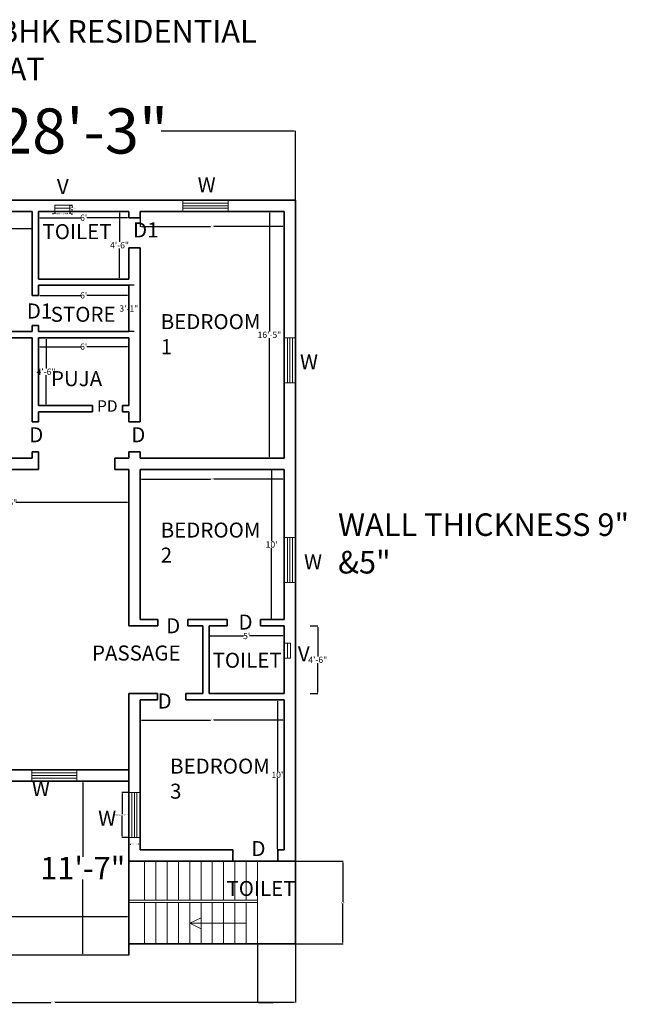
# Model space of a CAD drawing. Units: inches. Extents: x -304 to 580, y 363 to 1149.
# Tile 11 of 11: x 96 to 580, y 363 to 1149. Entities that reach past the tile are written whole.
import ezdxf

# ---------------------------------------------------------------- set-up
doc = ezdxf.new("R2010")
doc.units = ezdxf.units.IN
doc.header["$MEASUREMENT"] = 0
for name, color, linetype, lineweight in [('A-ANNO-DIMS', 2, 'Continuous', 13), ('A-ANNO-IDEN', 7, 'Continuous', 18), ('A-ANNO-SYMB', 7, 'Continuous', 18), ('A-ANNO-TEXT', 7, 'Continuous', 25), ('A-AREA-IDEN', 7, 'Continuous', 25), ('A-FLOR-OTLN', 2, 'Continuous', 25), ('A-FLOR-STRS', 40, 'Continuous', 18), ('A-GLAZ', 4, 'Continuous', 18), ('A-GLAZ-VENT', 4, 'Continuous', 18), ('A-WALL', 40, 'Continuous', 35)]:
    doc.layers.add(name, color=color, linetype=linetype, lineweight=lineweight)
doc.styles.get("Standard").update_dxf_attribs({"font": 'arial.ttf'})
doc.dimstyles.get("Standard").update_dxf_attribs({"dimtxt": 1, "dimasz": 1, "dimexe": 0.18, "dimexo": 0.0625, "dimgap": 0.09, "dimtad": 0, "dimtih": 1, "dimtoh": 1, "dimdec": 0, "dimzin": 0, "dimdsep": 46, "dimlunit": 3, "dimtxsty": 'Standard', "dimcen": 0.09, "dimadec": 0, "dimazin": 0, "dimtfac": 1, "dimtdec": 0, "dimtofl": 0, "dimtmove": 0, "dimatfit": 3, "dimfxl": 1, "dimtolj": 1, "dimtzin": 0, "dimarcsym": 0})

# ---------------------------------------------------------------- blocks, each defined once
blk = doc.blocks.new('*D2')
at = {"layer": 'A-ANNO-DIMS', "color": 0, "lineweight": -2, "transparency": 16777216}
for p, q in [((-22.57, 1005.01), (-22.57, 1060.38)), ((-21.57, 1060.2), (84.7, 1060.2)), ((315.43, 1060.2), (209.16, 1060.2)), ((316.43, 1005.01), (316.43, 1060.38))]:
    blk.add_line(p, q, dxfattribs=at)
at = {"layer": 'A-ANNO-DIMS', "color": 0, "transparency": 16777216}
for points in [[(-21.57, 1060.37), (-21.57, 1060.04), (-22.57, 1060.2)], [(315.43, 1060.37), (315.43, 1060.04), (316.43, 1060.2)]]:
    blk.add_solid(points, dxfattribs=at)
at = {"layer": 'Defpoints', "color": 0, "transparency": 16777216}
for p in [(316.43, 1060.2), (-22.57, 1004.95), (316.43, 1004.95)]:
    blk.add_point(p, dxfattribs=at)
at = {"layer": 'A-ANNO-DIMS', "color": 0, "transparency": 16777216, "insert": (146.93, 1060.2), "char_height": 1, "attachment_point": 5}
blk.add_mtext('\\A1;{\\H36x;28\'-3"}', dxfattribs=at)
blk = doc.blocks.new('*D4')
at = {"layer": 'A-ANNO-DIMS', "color": 0, "lineweight": -2, "transparency": 16777216}
for p, q in [((-13.57, 789.88), (-13.57, 763.24)), ((183.43, 789.88), (183.43, 763.24)), ((-12.57, 763.42), (76.49, 763.42)), ((182.43, 763.42), (93.37, 763.42))]:
    blk.add_line(p, q, dxfattribs=at)
at = {"layer": 'A-ANNO-DIMS', "color": 0, "transparency": 16777216}
for points in [[(-12.57, 763.59), (-12.57, 763.26), (-13.57, 763.42)], [(182.43, 763.59), (182.43, 763.26), (183.43, 763.42)]]:
    blk.add_solid(points, dxfattribs=at)
at = {"layer": 'Defpoints', "color": 0, "transparency": 16777216}
for p in [(-13.57, 789.95), (183.43, 789.95), (183.43, 763.42)]:
    blk.add_point(p, dxfattribs=at)
at = {"layer": 'A-ANNO-DIMS', "color": 0, "transparency": 16777216, "insert": (84.93, 763.42), "char_height": 1, "attachment_point": 5}
blk.add_mtext('\\A1;{\\H5x;16\'-5"}', dxfattribs=at)
blk = doc.blocks.new('*D5')
at = {"layer": 'A-ANNO-DIMS', "color": 0, "lineweight": -2, "transparency": 16777216}
for p, q in [((-13.57, 995.88), (-13.57, 981.84)), ((106.43, 995.88), (106.43, 981.84)), ((-12.57, 982.02), (42.33, 982.02)), ((105.43, 982.02), (50.53, 982.02))]:
    blk.add_line(p, q, dxfattribs=at)
at = {"layer": 'A-ANNO-DIMS', "color": 0, "transparency": 16777216}
for points in [[(-12.57, 982.19), (-12.57, 981.85), (-13.57, 982.02)], [(105.43, 982.19), (105.43, 981.85), (106.43, 982.02)]]:
    blk.add_solid(points, dxfattribs=at)
at = {"layer": 'Defpoints', "color": 0, "transparency": 16777216}
for p in [(-13.57, 995.95), (106.43, 995.95), (106.43, 982.02)]:
    blk.add_point(p, dxfattribs=at)
at = {"layer": 'A-ANNO-DIMS', "color": 0, "transparency": 16777216, "insert": (46.43, 982.02), "char_height": 1, "attachment_point": 5}
blk.add_mtext("\\A1;{\\H5x;10'}", dxfattribs=at)
blk = doc.blocks.new('*D7')
at = {"layer": 'A-ANNO-DIMS', "color": 0, "lineweight": -2, "transparency": 16777216}
for p, q in [((183.37, 995.95), (175.83, 995.95)), ((176.01, 994.95), (176.01, 971.59)), ((176.01, 942.95), (176.01, 966.3)), ((183.37, 941.95), (175.83, 941.95))]:
    blk.add_line(p, q, dxfattribs=at)
at = {"layer": 'A-ANNO-DIMS', "color": 0, "transparency": 16777216}
for points in [[(175.84, 994.95), (176.17, 994.95), (176.01, 995.95)], [(175.84, 942.95), (176.17, 942.95), (176.01, 941.95)]]:
    blk.add_solid(points, dxfattribs=at)
at = {"layer": 'Defpoints', "color": 0, "transparency": 16777216}
for p in [(183.43, 995.95), (176.01, 941.95), (183.43, 941.95)]:
    blk.add_point(p, dxfattribs=at)
at = {"layer": 'A-ANNO-DIMS', "color": 0, "transparency": 16777216, "insert": (176.01, 968.95), "char_height": 1, "attachment_point": 5}
blk.add_mtext('\\A1;{\\H5x;4\'-6"}', dxfattribs=at)
blk = doc.blocks.new('*D8')
at = {"layer": 'A-ANNO-DIMS', "color": 0, "lineweight": -2, "transparency": 16777216}
for p, q in [((111.43, 995.88), (111.43, 990.77)), ((112.43, 990.95), (145.03, 990.95)), ((182.43, 990.95), (149.83, 990.95)), ((183.43, 995.88), (183.43, 990.77))]:
    blk.add_line(p, q, dxfattribs=at)
at = {"layer": 'A-ANNO-DIMS', "color": 0, "transparency": 16777216}
for points in [[(112.43, 991.11), (112.43, 990.78), (111.43, 990.95)], [(182.43, 991.11), (182.43, 990.78), (183.43, 990.95)]]:
    blk.add_solid(points, dxfattribs=at)
at = {"layer": 'Defpoints', "color": 0, "transparency": 16777216}
for p in [(111.43, 995.95), (183.43, 995.95), (183.43, 990.95)]:
    blk.add_point(p, dxfattribs=at)
at = {"layer": 'A-ANNO-DIMS', "color": 0, "transparency": 16777216, "insert": (147.43, 990.95), "char_height": 1, "attachment_point": 5}
blk.add_mtext("\\A1;{\\H5x;6'}", dxfattribs=at)
blk = doc.blocks.new('*D9')
at = {"layer": 'A-ANNO-DIMS', "color": 0, "lineweight": -2, "transparency": 16777216}
for p, q in [((192.43, 995.88), (192.43, 983.76)), ((307.43, 995.88), (307.43, 983.76)), ((193.43, 983.94), (248.51, 983.94)), ((306.43, 983.94), (251.35, 983.94))]:
    blk.add_line(p, q, dxfattribs=at)
at = {"layer": 'A-ANNO-DIMS', "color": 0, "transparency": 16777216}
for points in [[(193.43, 984.1), (193.43, 983.77), (192.43, 983.94)], [(306.43, 984.1), (306.43, 983.77), (307.43, 983.94)]]:
    blk.add_solid(points, dxfattribs=at)
at = {"layer": 'Defpoints', "color": 0, "transparency": 16777216}
for p in [(192.43, 995.95), (307.43, 995.95), (307.43, 983.94)]:
    blk.add_point(p, dxfattribs=at)
at = {"layer": 'A-ANNO-DIMS', "color": 0, "transparency": 16777216, "insert": (249.93, 983.94), "char_height": 1, "attachment_point": 5}
blk.add_mtext('\\A1;9\'-7"', dxfattribs=at)
blk = doc.blocks.new('*D10')
at = {"layer": 'A-ANNO-DIMS', "color": 0, "lineweight": -2, "transparency": 16777216}
for p, q in [((307.37, 995.95), (295.43, 995.95)), ((295.61, 994.95), (295.61, 900.09)), ((295.61, 799.95), (295.61, 894.8)), ((307.37, 798.95), (295.43, 798.95))]:
    blk.add_line(p, q, dxfattribs=at)
at = {"layer": 'A-ANNO-DIMS', "color": 0, "transparency": 16777216}
for points in [[(295.44, 994.95), (295.77, 994.95), (295.61, 995.95)], [(295.44, 799.95), (295.77, 799.95), (295.61, 798.95)]]:
    blk.add_solid(points, dxfattribs=at)
at = {"layer": 'Defpoints', "color": 0, "transparency": 16777216}
for p in [(307.43, 995.95), (295.61, 798.95), (307.43, 798.95)]:
    blk.add_point(p, dxfattribs=at)
at = {"layer": 'A-ANNO-DIMS', "color": 0, "transparency": 16777216, "insert": (295.61, 897.45), "char_height": 1, "attachment_point": 5}
blk.add_mtext('\\A1;{\\H5x;16\'-5"}', dxfattribs=at)
blk = doc.blocks.new('*D11')
at = {"layer": 'A-ANNO-DIMS', "color": 0, "lineweight": -2, "transparency": 16777216}
for p, q in [((192.43, 789.88), (192.43, 782.02)), ((307.43, 789.88), (307.43, 782.02)), ((193.43, 782.2), (248.51, 782.2)), ((306.43, 782.2), (251.35, 782.2))]:
    blk.add_line(p, q, dxfattribs=at)
at = {"layer": 'A-ANNO-DIMS', "color": 0, "transparency": 16777216}
for points in [[(193.43, 782.37), (193.43, 782.04), (192.43, 782.2)], [(306.43, 782.37), (306.43, 782.04), (307.43, 782.2)]]:
    blk.add_solid(points, dxfattribs=at)
at = {"layer": 'Defpoints', "color": 0, "transparency": 16777216}
for p in [(192.43, 789.95), (307.43, 789.95), (307.43, 782.2)]:
    blk.add_point(p, dxfattribs=at)
at = {"layer": 'A-ANNO-DIMS', "color": 0, "transparency": 16777216, "insert": (249.93, 782.2), "char_height": 1, "attachment_point": 5}
blk.add_mtext('\\A1;9\'-7"', dxfattribs=at)
blk = doc.blocks.new('*D12')
at = {"layer": 'A-ANNO-DIMS', "color": 0, "lineweight": -2, "transparency": 16777216}
for p, q in [((307.37, 789.95), (297.18, 789.95)), ((297.36, 788.95), (297.36, 732.59)), ((297.36, 670.95), (297.36, 727.3)), ((307.37, 669.95), (297.18, 669.95))]:
    blk.add_line(p, q, dxfattribs=at)
at = {"layer": 'A-ANNO-DIMS', "color": 0, "transparency": 16777216}
for points in [[(297.19, 788.95), (297.53, 788.95), (297.36, 789.95)], [(297.19, 670.95), (297.53, 670.95), (297.36, 669.95)]]:
    blk.add_solid(points, dxfattribs=at)
at = {"layer": 'Defpoints', "color": 0, "transparency": 16777216}
for p in [(307.43, 789.95), (297.36, 669.95), (307.43, 669.95)]:
    blk.add_point(p, dxfattribs=at)
at = {"layer": 'A-ANNO-DIMS', "color": 0, "transparency": 16777216, "insert": (297.36, 729.95), "char_height": 1, "attachment_point": 5}
blk.add_mtext("\\A1;{\\H5x;10'}", dxfattribs=at)
blk = doc.blocks.new('*D13')
at = {"layer": 'A-ANNO-DIMS', "color": 0, "lineweight": -2, "transparency": 16777216}
for p, q in [((307.37, 605.95), (301.81, 605.95)), ((301.99, 604.95), (301.99, 548.59)), ((301.99, 486.95), (301.99, 543.3)), ((307.37, 485.95), (301.81, 485.95))]:
    blk.add_line(p, q, dxfattribs=at)
at = {"layer": 'A-ANNO-DIMS', "color": 0, "transparency": 16777216}
for points in [[(301.82, 604.95), (302.16, 604.95), (301.99, 605.95)], [(301.82, 486.95), (302.16, 486.95), (301.99, 485.95)]]:
    blk.add_solid(points, dxfattribs=at)
at = {"layer": 'Defpoints', "color": 0, "transparency": 16777216}
for p in [(307.43, 605.95), (301.99, 485.95), (307.43, 485.95)]:
    blk.add_point(p, dxfattribs=at)
at = {"layer": 'A-ANNO-DIMS', "color": 0, "transparency": 16777216, "insert": (301.99, 545.95), "char_height": 1, "attachment_point": 5}
blk.add_mtext("\\A1;{\\H5x;10'}", dxfattribs=at)
blk = doc.blocks.new('*D14')
at = {"layer": 'A-ANNO-DIMS', "color": 0, "lineweight": -2, "transparency": 16777216}
for p, q in [((192.43, 604.88), (192.43, 589.47)), ((307.43, 604.88), (307.43, 589.47)), ((193.43, 589.65), (248.51, 589.65)), ((306.43, 589.65), (251.35, 589.65))]:
    blk.add_line(p, q, dxfattribs=at)
at = {"layer": 'A-ANNO-DIMS', "color": 0, "transparency": 16777216}
for points in [[(193.43, 589.82), (193.43, 589.48), (192.43, 589.65)], [(306.43, 589.82), (306.43, 589.48), (307.43, 589.65)]]:
    blk.add_solid(points, dxfattribs=at)
at = {"layer": 'Defpoints', "color": 0, "transparency": 16777216}
for p in [(192.43, 604.95), (307.43, 604.95), (192.43, 589.65)]:
    blk.add_point(p, dxfattribs=at)
at = {"layer": 'A-ANNO-DIMS', "color": 0, "transparency": 16777216, "insert": (249.93, 589.65), "char_height": 1, "attachment_point": 5}
blk.add_mtext('\\A1;9\'-7"', dxfattribs=at)
blk = doc.blocks.new('*D15')
at = {"layer": 'A-ANNO-DIMS', "color": 0, "lineweight": -2, "transparency": 16777216}
for p, q in [((111.43, 894.88), (111.43, 887.76)), ((183.43, 894.88), (183.43, 887.76)), ((112.43, 887.94), (145.03, 887.94)), ((182.43, 887.94), (149.83, 887.94))]:
    blk.add_line(p, q, dxfattribs=at)
at = {"layer": 'A-ANNO-DIMS', "color": 0, "transparency": 16777216}
for points in [[(112.43, 888.11), (112.43, 887.77), (111.43, 887.94)], [(182.43, 888.11), (182.43, 887.77), (183.43, 887.94)]]:
    blk.add_solid(points, dxfattribs=at)
at = {"layer": 'Defpoints', "color": 0, "transparency": 16777216}
for p in [(111.43, 894.95), (183.43, 894.95), (183.43, 887.94)]:
    blk.add_point(p, dxfattribs=at)
at = {"layer": 'A-ANNO-DIMS', "color": 0, "transparency": 16777216, "insert": (147.43, 887.94), "char_height": 1, "attachment_point": 5}
blk.add_mtext("\\A1;{\\H5x;6'}", dxfattribs=at)
blk = doc.blocks.new('*D16')
at = {"layer": 'A-ANNO-DIMS', "color": 0, "lineweight": -2, "transparency": 16777216}
for p, q in [((111.49, 894.95), (117.53, 894.95)), ((117.35, 893.95), (117.35, 870.59)), ((117.35, 841.95), (117.35, 865.3)), ((111.49, 840.95), (117.53, 840.95))]:
    blk.add_line(p, q, dxfattribs=at)
at = {"layer": 'A-ANNO-DIMS', "color": 0, "transparency": 16777216}
for points in [[(117.19, 893.95), (117.52, 893.95), (117.35, 894.95)], [(117.19, 841.95), (117.52, 841.95), (117.35, 840.95)]]:
    blk.add_solid(points, dxfattribs=at)
at = {"layer": 'Defpoints', "color": 0, "transparency": 16777216}
for p in [(111.43, 894.95), (117.35, 894.95), (111.43, 840.95)]:
    blk.add_point(p, dxfattribs=at)
at = {"layer": 'A-ANNO-DIMS', "color": 0, "transparency": 16777216, "insert": (117.35, 867.95), "char_height": 1, "attachment_point": 5}
blk.add_mtext('\\A1;{\\H5x;4\'-6"}', dxfattribs=at)
blk = doc.blocks.new('*D17')
at = {"layer": 'A-ANNO-DIMS', "color": 0, "lineweight": -2, "transparency": 16777216}
for p, q in [((328.17, 664.86), (334.34, 664.86)), ((334.16, 663.86), (334.16, 640.5)), ((334.16, 611.86), (334.16, 635.21)), ((328.17, 610.86), (334.34, 610.86))]:
    blk.add_line(p, q, dxfattribs=at)
at = {"layer": 'A-ANNO-DIMS', "color": 0, "transparency": 16777216}
for points in [[(334, 663.86), (334.33, 663.86), (334.16, 664.86)], [(334, 611.86), (334.33, 611.86), (334.16, 610.86)]]:
    blk.add_solid(points, dxfattribs=at)
at = {"layer": 'Defpoints', "color": 0, "transparency": 16777216}
for p in [(328.11, 664.86), (328.11, 610.86), (334.16, 610.86)]:
    blk.add_point(p, dxfattribs=at)
at = {"layer": 'A-ANNO-DIMS', "color": 0, "transparency": 16777216, "insert": (334.16, 637.86), "char_height": 1, "attachment_point": 5}
blk.add_mtext('\\A1;{\\H5x;4\'-6"}', dxfattribs=at)
blk = doc.blocks.new('*D18')
at = {"layer": 'A-ANNO-DIMS', "color": 0, "lineweight": -2, "transparency": 16777216}
for p, q in [((247.43, 664.88), (247.43, 656.7)), ((307.43, 664.88), (307.43, 656.7)), ((248.43, 656.88), (275.04, 656.88)), ((306.43, 656.88), (279.82, 656.88))]:
    blk.add_line(p, q, dxfattribs=at)
at = {"layer": 'A-ANNO-DIMS', "color": 0, "transparency": 16777216}
for points in [[(248.43, 657.05), (248.43, 656.71), (247.43, 656.88)], [(306.43, 657.05), (306.43, 656.71), (307.43, 656.88)]]:
    blk.add_solid(points, dxfattribs=at)
at = {"layer": 'Defpoints', "color": 0, "transparency": 16777216}
for p in [(247.43, 664.95), (307.43, 664.95), (307.43, 656.88)]:
    blk.add_point(p, dxfattribs=at)
at = {"layer": 'A-ANNO-DIMS', "color": 0, "transparency": 16777216, "insert": (277.43, 656.88), "char_height": 1, "attachment_point": 5}
blk.add_mtext("\\A1;{\\H5x;5'}", dxfattribs=at)
blk = doc.blocks.new('*D19')
at = {"layer": 'A-ANNO-DIMS', "color": 0, "lineweight": -2, "transparency": 16777216}
for p, q in [((187.82, 936.95), (183.25, 936.95)), ((183.43, 935.95), (183.43, 921.09)), ((183.43, 900.95), (183.43, 915.8)), ((187.82, 899.95), (183.25, 899.95))]:
    blk.add_line(p, q, dxfattribs=at)
at = {"layer": 'A-ANNO-DIMS', "color": 0, "transparency": 16777216}
for points in [[(183.26, 935.95), (183.6, 935.95), (183.43, 936.95)], [(183.26, 900.95), (183.6, 900.95), (183.43, 899.95)]]:
    blk.add_solid(points, dxfattribs=at)
at = {"layer": 'Defpoints', "color": 0, "transparency": 16777216}
for p in [(187.88, 936.95), (183.43, 899.95), (187.88, 899.95)]:
    blk.add_point(p, dxfattribs=at)
at = {"layer": 'A-ANNO-DIMS', "color": 0, "transparency": 16777216, "insert": (183.43, 918.45), "char_height": 1, "attachment_point": 5}
blk.add_mtext('\\A1;{\\H5x;3\'-1"}', dxfattribs=at)
blk = doc.blocks.new('*D20')
at = {"layer": 'A-ANNO-DIMS', "color": 0, "lineweight": -2, "transparency": 16777216}
for p, q in [((111.43, 936.88), (111.43, 928.77)), ((183.43, 936.88), (183.43, 928.77)), ((112.43, 928.95), (145.03, 928.95)), ((182.43, 928.95), (149.83, 928.95))]:
    blk.add_line(p, q, dxfattribs=at)
at = {"layer": 'A-ANNO-DIMS', "color": 0, "transparency": 16777216}
for points in [[(112.43, 929.11), (112.43, 928.78), (111.43, 928.95)], [(182.43, 929.11), (182.43, 928.78), (183.43, 928.95)]]:
    blk.add_solid(points, dxfattribs=at)
at = {"layer": 'Defpoints', "color": 0, "transparency": 16777216}
for p in [(111.43, 936.95), (183.43, 936.95), (111.43, 928.95)]:
    blk.add_point(p, dxfattribs=at)
at = {"layer": 'A-ANNO-DIMS', "color": 0, "transparency": 16777216, "insert": (147.43, 928.95), "char_height": 1, "attachment_point": 5}
blk.add_mtext("\\A1;{\\H5x;6'}", dxfattribs=at)
blk = doc.blocks.new('*D21')
at = {"layer": 'A-ANNO-DIMS', "color": 0, "lineweight": -2, "transparency": 16777216}
for p, q in [((183.37, 540.95), (146.51, 540.95)), ((146.69, 539.95), (146.69, 480.57)), ((146.69, 402.95), (146.69, 462.32)), ((183.37, 401.95), (146.51, 401.95))]:
    blk.add_line(p, q, dxfattribs=at)
at = {"layer": 'A-ANNO-DIMS', "color": 0, "transparency": 16777216}
for points in [[(146.52, 539.95), (146.86, 539.95), (146.69, 540.95)], [(146.52, 402.95), (146.86, 402.95), (146.69, 401.95)]]:
    blk.add_solid(points, dxfattribs=at)
at = {"layer": 'Defpoints', "color": 0, "transparency": 16777216}
for p in [(183.43, 540.95), (146.69, 401.95), (183.43, 401.95)]:
    blk.add_point(p, dxfattribs=at)
at = {"layer": 'A-ANNO-DIMS', "color": 0, "transparency": 16777216, "insert": (146.69, 471.45), "char_height": 1, "attachment_point": 5}
blk.add_mtext('\\A1;{\\H18x;11\'-7"}', dxfattribs=at)
blk = doc.blocks.new('*D22')
at = {"layer": 'A-ANNO-DIMS', "color": 0, "lineweight": -2, "transparency": 16777216}
for p, q in [((-70.57, 402.01), (-70.57, 432.73)), ((-69.57, 432.55), (25.27, 432.55)), ((182.43, 432.55), (87.59, 432.55)), ((183.43, 402.01), (183.43, 432.73))]:
    blk.add_line(p, q, dxfattribs=at)
at = {"layer": 'A-ANNO-DIMS', "color": 0, "transparency": 16777216}
for points in [[(-69.57, 432.72), (-69.57, 432.38), (-70.57, 432.55)], [(182.43, 432.72), (182.43, 432.38), (183.43, 432.55)]]:
    blk.add_solid(points, dxfattribs=at)
at = {"layer": 'Defpoints', "color": 0, "transparency": 16777216}
for p in [(183.43, 432.55), (-70.57, 401.95), (183.43, 401.95)]:
    blk.add_point(p, dxfattribs=at)
at = {"layer": 'A-ANNO-DIMS', "color": 0, "transparency": 16777216, "insert": (56.43, 432.55), "char_height": 1, "attachment_point": 5}
blk.add_mtext('\\A1;{\\H18x;21\'-2"}', dxfattribs=at)
blk = doc.blocks.new('WIN-36IN')
for p, q in [((0, 6.5), (36, 6.5)), ((0, 4.5), (36, 4.5)), ((0, 2.5), (36, 2.5))]:
    blk.add_line(p, q)
blk.add_lwpolyline([(0, 0), (0, 9), (36, 9), (36, 0)], close=True)
blk = doc.blocks.new('VENT-12IN')
blk.add_line((0, 2.5), (12, 2.5))
blk.add_lwpolyline([(0, 0), (0, 5), (12, 5), (12, 0)], close=True)
blk = doc.blocks.new('*D25')
at = {"layer": 'A-ANNO-DIMS', "color": 0, "lineweight": -2, "transparency": 16777216}
for p, q in [((183.37, 531.97), (177.85, 531.97)), ((178.03, 530.97), (178.03, 514.58)), ((178.03, 496.97), (178.03, 513.36)), ((183.37, 495.97), (177.85, 495.97))]:
    blk.add_line(p, q, dxfattribs=at)
at = {"layer": 'A-ANNO-DIMS', "color": 0, "transparency": 16777216}
for points in [[(177.86, 530.97), (178.2, 530.97), (178.03, 531.97)], [(177.86, 496.97), (178.2, 496.97), (178.03, 495.97)]]:
    blk.add_solid(points, dxfattribs=at)
at = {"layer": 'Defpoints', "color": 0, "transparency": 16777216}
for p in [(183.43, 531.97), (178.03, 495.97), (183.43, 495.97)]:
    blk.add_point(p, dxfattribs=at)
at = {"layer": 'A-ANNO-DIMS', "color": 0, "transparency": 16777216, "insert": (178.03, 513.97), "char_height": 1, "attachment_point": 5}
blk.add_mtext('\\A1;WINDOW 3\'-0" TYP.', dxfattribs=at)
blk = doc.blocks.new('*D26')
at = {"layer": 'A-ANNO-DIMS', "color": 0, "lineweight": -2, "transparency": 16777216}
for p, q in [((183.43, 495.91), (183.43, 490.39)), ((192.43, 495.91), (192.43, 490.39)), ((184.43, 490.57), (184.79, 490.57)), ((191.43, 490.57), (191.07, 490.57))]:
    blk.add_line(p, q, dxfattribs=at)
at = {"layer": 'A-ANNO-DIMS', "color": 0, "transparency": 16777216}
for points in [[(184.43, 490.74), (184.43, 490.41), (183.43, 490.57)], [(191.43, 490.74), (191.43, 490.41), (192.43, 490.57)]]:
    blk.add_solid(points, dxfattribs=at)
at = {"layer": 'Defpoints', "color": 0, "transparency": 16777216}
for p in [(183.43, 495.97), (192.43, 495.97), (192.43, 490.57)]:
    blk.add_point(p, dxfattribs=at)
at = {"layer": 'A-ANNO-DIMS', "color": 0, "transparency": 16777216, "insert": (187.93, 490.57), "char_height": 1, "attachment_point": 5}
blk.add_mtext('\\A1;0\'-9" TYP.', dxfattribs=at)
blk = doc.blocks.new('*D27')
at = {"layer": 'A-ANNO-DIMS', "color": 0, "lineweight": -2, "transparency": 16777216}
for p, q in [((123.43, 994.14), (122.43, 994.14)), ((124.43, 995.87), (124.43, 993.96)), ((136.43, 995.87), (136.43, 993.96)), ((137.43, 994.14), (138.43, 994.14))]:
    blk.add_line(p, q, dxfattribs=at)
at = {"layer": 'A-ANNO-DIMS', "color": 0, "transparency": 16777216}
for points in [[(123.43, 994.3), (123.43, 993.97), (124.43, 994.14)], [(137.43, 994.3), (137.43, 993.97), (136.43, 994.14)]]:
    blk.add_solid(points, dxfattribs=at)
at = {"layer": 'Defpoints', "color": 0, "transparency": 16777216}
for p in [(124.43, 995.94), (136.43, 995.94), (136.43, 994.14)]:
    blk.add_point(p, dxfattribs=at)
at = {"layer": 'A-ANNO-DIMS', "color": 0, "transparency": 16777216, "insert": (130.43, 994.14), "char_height": 1, "attachment_point": 5}
blk.add_mtext('\\A1;VENT 1\'-0" TYP.', dxfattribs=at)
blk = doc.blocks.new('*D28')
at = {"layer": 'A-ANNO-DIMS', "color": 0, "lineweight": -2, "transparency": 16777216}
for p, q in [((136.5, 1000.94), (138.41, 1000.94)), ((138.23, 999.94), (138.23, 999.04)), ((136.5, 995.94), (138.41, 995.94)), ((138.23, 996.94), (138.23, 997.84))]:
    blk.add_line(p, q, dxfattribs=at)
at = {"layer": 'A-ANNO-DIMS', "color": 0, "transparency": 16777216}
for points in [[(138.07, 999.94), (138.4, 999.94), (138.23, 1000.94)], [(138.07, 996.94), (138.4, 996.94), (138.23, 995.94)]]:
    blk.add_solid(points, dxfattribs=at)
at = {"layer": 'Defpoints', "color": 0, "transparency": 16777216}
for p in [(136.43, 1000.94), (138.23, 1000.94), (136.43, 995.94)]:
    blk.add_point(p, dxfattribs=at)
at = {"layer": 'A-ANNO-DIMS', "color": 0, "transparency": 16777216, "insert": (138.23, 998.44), "char_height": 1, "attachment_point": 5}
blk.add_mtext('\\A1;0\'-5" TYP.', dxfattribs=at)
blk = doc.blocks.new('*D29')
at = {"layer": 'A-ANNO-DIMS', "color": 0, "lineweight": -2, "transparency": 16777216}
for p, q in [((316.43, 410.88), (316.43, 364.02)), ((-70.57, 401.88), (-70.57, 364.02)), ((-69.57, 364.2), (121.12, 364.2)), ((315.43, 364.2), (124.74, 364.2))]:
    blk.add_line(p, q, dxfattribs=at)
at = {"layer": 'A-ANNO-DIMS', "color": 0, "transparency": 16777216}
for points in [[(-69.57, 364.36), (-69.57, 364.03), (-70.57, 364.2)], [(315.43, 364.36), (315.43, 364.03), (316.43, 364.2)]]:
    blk.add_solid(points, dxfattribs=at)
at = {"layer": 'Defpoints', "color": 0, "transparency": 16777216}
for p in [(316.43, 410.95), (-70.57, 401.95), (316.43, 364.2)]:
    blk.add_point(p, dxfattribs=at)
at = {"layer": 'A-ANNO-DIMS', "color": 0, "transparency": 16777216, "insert": (122.93, 364.2), "char_height": 1, "attachment_point": 5}
blk.add_mtext('\\A1;32\'-3"', dxfattribs=at)
blk = doc.blocks.new('*D31')
at = {"layer": 'A-ANNO-DIMS', "color": 0, "lineweight": -2, "transparency": 16777216}
for p, q in [((316.49, 476.95), (354.36, 476.95)), ((354.18, 475.95), (354.18, 444.55)), ((354.18, 411.95), (354.18, 443.35)), ((316.49, 410.95), (354.36, 410.95))]:
    blk.add_line(p, q, dxfattribs=at)
at = {"layer": 'A-ANNO-DIMS', "color": 0, "transparency": 16777216}
for points in [[(354.01, 475.95), (354.35, 475.95), (354.18, 476.95)], [(354.01, 411.95), (354.35, 411.95), (354.18, 410.95)]]:
    blk.add_solid(points, dxfattribs=at)
at = {"layer": 'Defpoints', "color": 0, "transparency": 16777216}
for p in [(316.43, 476.95), (354.18, 476.95), (316.43, 410.95)]:
    blk.add_point(p, dxfattribs=at)
at = {"layer": 'A-ANNO-DIMS', "color": 0, "transparency": 16777216, "insert": (354.18, 443.95), "char_height": 1, "attachment_point": 5}
blk.add_mtext('\\A1;5\'-6"', dxfattribs=at)
blk = doc.blocks.new('*D32')
at = {"layer": 'A-ANNO-DIMS', "color": 0, "lineweight": -2, "transparency": 16777216}
for p, q in [((286.03, 410.88), (286.03, 364.02)), ((316.43, 410.88), (316.43, 364.02)), ((287.03, 364.2), (298.64, 364.2)), ((315.43, 364.2), (303.82, 364.2))]:
    blk.add_line(p, q, dxfattribs=at)
at = {"layer": 'A-ANNO-DIMS', "color": 0, "transparency": 16777216}
for points in [[(287.03, 364.36), (287.03, 364.03), (286.03, 364.2)], [(315.43, 364.36), (315.43, 364.03), (316.43, 364.2)]]:
    blk.add_solid(points, dxfattribs=at)
at = {"layer": 'Defpoints', "color": 0, "transparency": 16777216}
for p in [(286.03, 410.95), (316.43, 410.95), (316.43, 364.2)]:
    blk.add_point(p, dxfattribs=at)
at = {"layer": 'A-ANNO-DIMS', "color": 0, "transparency": 16777216, "insert": (301.23, 364.2), "char_height": 1, "attachment_point": 5}
blk.add_mtext('\\A1;2\'-6 1/2"', dxfattribs=at)
blk = doc.blocks.new('*D33')
at = {"layer": 'A-ANNO-DIMS', "color": 0, "lineweight": -2, "transparency": 16777216}
for p, q in [((106.37, 894.95), (-108.5, 894.95)), ((-108.32, 893.95), (-108.32, 847.55)), ((-108.32, 799.95), (-108.32, 846.35)), ((106.37, 798.95), (-108.5, 798.95))]:
    blk.add_line(p, q, dxfattribs=at)
at = {"layer": 'A-ANNO-DIMS', "color": 0, "transparency": 16777216}
for points in [[(-108.49, 893.95), (-108.15, 893.95), (-108.32, 894.95)], [(-108.49, 799.95), (-108.15, 799.95), (-108.32, 798.95)]]:
    blk.add_solid(points, dxfattribs=at)
at = {"layer": 'Defpoints', "color": 0, "transparency": 16777216}
for p in [(-108.32, 894.95), (106.43, 894.95), (106.43, 798.95)]:
    blk.add_point(p, dxfattribs=at)
at = {"layer": 'A-ANNO-DIMS', "color": 0, "transparency": 16777216, "insert": (-108.32, 846.95), "char_height": 1, "attachment_point": 5}
blk.add_mtext('\\A1;8\'-0"', dxfattribs=at)

msp = doc.modelspace()

# ---------------------------------------------------------------- linework, layer by layer
at = {"layer": 'A-ANNO-SYMB'}
for p, q in [((232.03, 427.45), (241.03, 431.83)), ((277.03, 427.45), (232.03, 427.45)), ((241.03, 423.02), (232.03, 427.45)), ((241.03, 431.83), (241.03, 423.02))]:
    msp.add_line(p, q, dxfattribs=at)
at = {"layer": 'A-FLOR-OTLN'}
msp.add_line((183.43, 401.95), (-70.57, 401.95), dxfattribs=at)
at = {"layer": 'A-FLOR-STRS'}
for p, q in [((196.03, 476.95), (196.03, 445.95)), ((205.03, 476.95), (205.03, 445.95)), ((214.03, 476.95), (214.03, 445.95)), ((223.03, 476.95), (223.03, 445.95)), ((232.03, 476.95), (232.03, 445.95)), ((241.03, 476.95), (241.03, 445.95)), ((241.03, 476.95), (241.03, 445.95)), ((250.03, 476.95), (250.03, 445.95)), ((259.03, 476.95), (259.03, 445.95)), ((268.03, 476.95), (268.03, 445.95)), ((268.03, 476.95), (268.03, 445.95)), ((277.03, 476.95), (277.03, 445.95)), ((286.03, 476.95), (286.03, 410.95)), ((286.03, 445.95), (183.43, 445.95)), ((286.03, 443.95), (183.43, 443.95)), ((196.03, 443.95), (196.03, 410.95)), ((205.03, 443.95), (205.03, 410.95)), ((214.03, 443.95), (214.03, 410.95)), ((223.03, 443.95), (223.03, 410.95)), ((232.03, 443.95), (232.03, 410.95)), ((241.03, 443.95), (241.03, 410.95)), ((241.03, 443.95), (241.03, 410.95)), ((250.03, 443.95), (250.03, 410.95)), ((259.03, 443.95), (259.03, 410.95)), ((268.03, 443.95), (268.03, 410.95)), ((268.03, 443.95), (268.03, 410.95)), ((277.03, 443.95), (277.03, 410.95))]:
    msp.add_line(p, q, dxfattribs=at)
at = {"layer": 'A-WALL'}
for p, q in [((-22.57, 1004.95), (316.43, 1004.95)), ((316.43, 1004.95), (316.43, 410.95)), ((-13.57, 995.95), (106.43, 995.95)), ((106.43, 928.95), (106.43, 995.95)), ((111.43, 995.95), (183.43, 995.95)), ((111.43, 941.95), (111.43, 995.95)), ((183.43, 990.95), (183.43, 995.95)), ((183.43, 990.95), (192.43, 990.95)), ((192.43, 995.95), (307.43, 995.95)), ((192.43, 990.95), (192.43, 995.95)), ((307.43, 995.95), (307.43, 798.95)), ((183.43, 941.95), (183.43, 966.95)), ((183.43, 966.95), (192.43, 966.95)), ((192.43, 827.95), (192.43, 966.95)), ((111.43, 941.95), (183.43, 941.95)), ((111.43, 936.95), (183.43, 936.95)), ((111.43, 928.95), (111.43, 936.95)), ((183.43, 899.95), (183.43, 936.95)), ((111.43, 928.95), (106.43, 928.95)), ((106.43, 899.95), (106.43, 904.95)), ((111.43, 904.95), (106.43, 904.95)), ((111.43, 899.95), (111.43, 904.95)), ((27.43, 899.95), (106.43, 899.95)), ((111.43, 899.95), (183.43, 899.95)), ((27.43, 894.95), (106.43, 894.95)), ((106.43, 827.95), (106.43, 894.95)), ((111.43, 894.95), (183.43, 894.95)), ((111.43, 840.95), (111.43, 894.95)), ((183.43, 840.95), (183.43, 894.95)), ((111.43, 840.95), (154.43, 840.95)), ((111.43, 835.95), (154.43, 835.95)), ((111.43, 827.95), (111.43, 835.95)), ((154.43, 835.95), (154.43, 840.95)), ((178.43, 835.95), (178.43, 840.95)), ((178.43, 840.95), (183.43, 840.95)), ((178.43, 835.95), (183.43, 835.95)), ((183.43, 827.95), (183.43, 835.95)), ((106.43, 827.95), (111.43, 827.95)), ((192.43, 827.95), (183.43, 827.95)), ((106.43, 798.95), (106.43, 803.95)), ((106.43, 803.95), (111.43, 803.95)), ((111.43, 789.95), (111.43, 803.95)), ((192.43, 803.95), (183.43, 803.95)), ((183.43, 798.95), (183.43, 803.95)), ((192.43, 798.95), (192.43, 803.95)), ((-13.57, 798.95), (106.43, 798.95)), ((172.14, 798.95), (183.43, 798.95)), ((172.14, 789.95), (172.14, 798.95)), ((192.43, 798.95), (307.43, 798.95)), ((-13.57, 789.95), (111.43, 789.95)), ((172.14, 789.95), (183.43, 789.95)), ((183.43, 664.95), (183.43, 789.95)), ((192.43, 669.95), (192.43, 789.95)), ((192.43, 789.95), (307.43, 789.95)), ((307.43, 789.95), (307.43, 669.95)), ((192.43, 669.95), (206.49, 669.95)), ((206.49, 669.95), (206.49, 664.95)), ((230.58, 669.95), (230.58, 664.95)), ((230.58, 669.95), (261.81, 669.95)), ((261.81, 669.95), (261.81, 664.95)), ((288.47, 669.95), (288.47, 664.95)), ((288.47, 669.95), (307.43, 669.95)), ((183.43, 664.95), (206.49, 664.95)), ((230.58, 664.95), (242.43, 664.95)), ((242.43, 664.95), (242.43, 610.95)), ((247.43, 664.95), (247.43, 610.95)), ((247.43, 664.95), (261.81, 664.95)), ((288.47, 664.95), (307.43, 664.95)), ((307.43, 664.95), (307.43, 610.95)), ((183.43, 401.95), (183.43, 610.95)), ((183.43, 610.95), (206.36, 610.95)), ((192.43, 605.95), (206.36, 605.95)), ((192.43, 485.95), (192.43, 605.95)), ((206.36, 610.95), (206.36, 605.95)), ((228.86, 610.95), (228.86, 605.95)), ((228.86, 610.95), (242.43, 610.95)), ((228.86, 605.95), (307.43, 605.95)), ((247.43, 610.95), (307.43, 610.95)), ((307.43, 605.95), (307.43, 485.95)), ((58.51, 549.95), (183.43, 549.95)), ((58.51, 540.95), (183.43, 540.95)), ((192.43, 485.95), (266.43, 485.95)), ((266.43, 485.95), (266.43, 476.95)), ((302.43, 485.95), (302.43, 476.95)), ((302.43, 485.95), (307.43, 485.95)), ((183.43, 476.95), (302.43, 476.95)), ((302.43, 476.95), (316.43, 476.95)), ((316.43, 410.95), (183.43, 410.95))]:
    msp.add_line(p, q, dxfattribs=at)

# ---------------------------------------------------------------- block references
at = {"layer": 'A-GLAZ'}
for p in [(226.63, 995.95), (106.08, 540.95)]:
    msp.add_blockref('WIN-36IN', p, dxfattribs=at)
for p, rotation in [((307.43, 895.08), 269.9999999999999), ((307.43, 735.67), 270.0000000000002), ((183.43, 531.97), 269.9999999999999)]:
    msp.add_blockref('WIN-36IN', p, dxfattribs=dict(at, rotation=rotation))
at = {"layer": 'A-GLAZ-VENT'}
msp.add_blockref('VENT-12IN', (124.43, 995.94), dxfattribs=at)
at = {"layer": 'A-GLAZ-VENT', "rotation": 270.0000000000011}
msp.add_blockref('VENT-12IN', (307.48, 651.21), dxfattribs=at)

# ---------------------------------------------------------------- texts
at = {"layer": 'A-ANNO-IDEN', "attachment_point": 1}
for s, width, gutter_width, insert, char_height in [('W', 41.6501, 1, (238.35, 1023.27), 12), ('V', 10.0311, 1, (126.03, 1021.76), 12), ('D1', 12.3109, 1, (186.8, 987.22), 12), ('D1', 12.3109, 1, (102.04, 922.43), 12), ('W', 41.6501, 1, (320, 881.84), 12), ('PD', 9.3512, 0.76, (158.04, 845.12), 9.115), ('D', 12.3109, 1, (103.94, 823.58), 12), ('D', 12.3109, 1, (185.38, 823.58), 12), ('W', 41.6501, 1, (323.22, 722.09), 12), ('D', 12.3109, 1, (213.21, 671.02), 12), ('D', 12.3109, 1, (270.96, 673.99), 12), ('V', 10.0311, 1, (318.32, 648.56), 12), ('D', 12.3109, 1, (206.36, 610.95), 12), ('W', 41.6501, 1, (106.08, 540.95), 12), ('W', 41.6501, 1, (158.97, 517.29), 12), ('D', 12.3109, 1, (281.26, 493.09), 12)]:
    msp.add_mtext_dynamic_manual_height_columns(s, width=width, gutter_width=gutter_width, heights=[0], dxfattribs=dict(at, insert=insert, char_height=char_height))
at = {"layer": 'A-ANNO-TEXT', "char_height": 18, "attachment_point": 1}
for s, width, insert in [('3 BHK RESIDENTIAL FLAT', 279.8589, (59.82, 1148.78)), ('WALL THICKNESS 9"\\P&5"', 275.8533, (350.37, 754.79))]:
    msp.add_mtext_dynamic_manual_height_columns(s, width=width, gutter_width=1, heights=[0], dxfattribs=dict(at, insert=insert))
at = {"layer": 'A-AREA-IDEN', "char_height": 12, "attachment_point": 1}
for s, width, insert in [('TOILET', 39.4169, (114.52, 985.82)), ('STORE', 39.4169, (121.11, 919.81)), ('BEDROOM\\P1', 79.7399, (208.88, 913.95)), ('PUJA', 39.4169, (121.28, 868.42)), ('BEDROOM\\P2', 79.7399, (208.88, 747.48)), ('PASSAGE', 39.4169, (154.04, 649.27)), ('TOILET', 39.4169, (250.26, 643.51)), ('BEDROOM\\P3', 79.7399, (216.34, 558.93)), ('TOILET', 39.4169, (261.33, 461.24))]:
    msp.add_mtext_dynamic_manual_height_columns(s, width=width, gutter_width=1, heights=[0], dxfattribs=dict(at, insert=insert))

# ---------------------------------------------------------------- dimensions: what is measured, and where the dimension line sits
at = {"layer": 'A-ANNO-DIMS'}
for base, p1, p2, text, override, picture, middle in [((316.43, 1060.2), (-22.57, 1004.95), (316.43, 1004.95), '{\\H36x;<>}', {"dimclrd": 0, "dimclre": 0, "dimclrt": 0}, '*D2', (146.93, 1060.2)), ((106.43, 982.02), (-13.57, 995.95), (106.43, 995.95), '{\\H5x;<>}', {"dimclrd": 0, "dimclre": 0, "dimclrt": 0}, '*D5', (46.43, 982.02)), ((183.43, 990.95), (111.43, 995.95), (183.43, 995.95), '{\\H5x;<>}', {"dimclrd": 0, "dimclre": 0, "dimclrt": 0}, '*D8', (147.43, 990.95)), ((136.43, 994.14), (124.43, 995.94), (136.43, 995.94), 'VENT <> TYP.', {"dimdec": 1, "dimlfac": 1, "dimrnd": 0, "dimzin": 1, "dimdsep": 46, "dimlunit": 4, "dimfrac": 2}, '*D27', (130.43, 994.14)), ((111.43, 928.95), (183.43, 936.95), (111.43, 936.95), '{\\H5x;<>}', {"dimclrd": 0, "dimclre": 0, "dimclrt": 0}, '*D20', (147.43, 928.95)), ((183.43, 887.94), (111.43, 894.95), (183.43, 894.95), '{\\H5x;<>}', {"dimclrd": 0, "dimclre": 0, "dimclrt": 0}, '*D15', (147.43, 887.94)), ((183.43, 763.42), (-13.57, 789.95), (183.43, 789.95), '{\\H5x;<>}', {"dimclrd": 0, "dimclre": 0, "dimclrt": 0}, '*D4', (84.93, 763.42)), ((307.43, 656.88), (247.43, 664.95), (307.43, 664.95), '{\\H5x;<>}', {"dimclrd": 0, "dimclre": 0, "dimclrt": 0}, '*D18', (277.43, 656.88)), ((192.43, 490.57), (183.43, 495.97), (192.43, 495.97), '<> TYP.', {"dimdec": 1, "dimlfac": 1, "dimrnd": 0, "dimzin": 1, "dimdsep": 46, "dimlunit": 4, "dimfrac": 2}, '*D26', (187.93, 490.57)), ((183.43, 432.55), (-70.57, 401.95), (183.43, 401.95), '{\\H18x;<>}', {"dimclrd": 0, "dimclre": 0, "dimclrt": 0}, '*D22', (56.43, 432.55))]:
    dim = msp.add_linear_dim(base=base, p1=p1, p2=p2, text=text, dimstyle='Standard', override=override, dxfattribs=at)
    dim.commit()
    dim.dimension.update_dxf_attribs({"geometry": picture, "text_midpoint": middle})
for base, p1, p2, angle, text, override, picture, middle in [((138.23, 1000.94), (136.43, 995.94), (136.43, 1000.94), 90, '<> TYP.', {"dimdec": 1, "dimlfac": 1, "dimrnd": 0, "dimzin": 1, "dimdsep": 46, "dimlunit": 4, "dimfrac": 2}, '*D28', (138.23, 998.44)), ((176.01, 941.95), (183.43, 995.95), (183.43, 941.95), 90, '{\\H5x;<>}', {"dimclrd": 0, "dimclre": 0, "dimclrt": 0}, '*D7', (176.01, 968.95)), ((295.61, 798.95), (307.43, 995.95), (307.43, 798.95), 90, '{\\H5x;<>}', {"dimclrd": 0, "dimclre": 0, "dimclrt": 0}, '*D10', (295.61, 897.45)), ((183.43, 899.95), (187.88, 936.95), (187.88, 899.95), 90, '{\\H5x;<>}', {"dimclrd": 0, "dimclre": 0, "dimclrt": 0}, '*D19', (183.43, 918.45)), ((117.35, 894.95), (111.43, 840.95), (111.43, 894.95), 90, '{\\H5x;<>}', {"dimclrd": 0, "dimclre": 0, "dimclrt": 0}, '*D16', (117.35, 867.95)), ((297.36, 669.95), (307.43, 789.95), (307.43, 669.95), 90, '{\\H5x;<>}', {"dimclrd": 0, "dimclre": 0, "dimclrt": 0}, '*D12', (297.36, 729.95)), ((334.16, 610.86), (328.11, 664.86), (328.11, 610.86), 90, '{\\H5x;<>}', {"dimclrd": 0, "dimclre": 0, "dimclrt": 0}, '*D17', (334.16, 637.86)), ((301.99, 485.95), (307.43, 605.95), (307.43, 485.95), 90, '{\\H5x;<>}', {"dimclrd": 0, "dimclre": 0, "dimclrt": 0}, '*D13', (301.99, 545.95)), ((146.69, 401.95), (183.43, 540.95), (183.43, 401.95), 90, '{\\H18x;<>}', {"dimclrd": 0, "dimclre": 0, "dimclrt": 0}, '*D21', (146.69, 471.45)), ((178.03, 495.97), (183.43, 531.97), (183.43, 495.97), 270, 'WINDOW <> TYP.', {"dimdec": 1, "dimlfac": 1, "dimrnd": 0, "dimzin": 1, "dimdsep": 46, "dimlunit": 4, "dimfrac": 2}, '*D25', (178.03, 513.97))]:
    dim = msp.add_linear_dim(base=base, p1=p1, p2=p2, angle=angle, text=text, dimstyle='Standard', override=override, dxfattribs=at)
    dim.commit()
    dim.dimension.update_dxf_attribs({"geometry": picture, "text_midpoint": middle})
for base, p1, p2, override, picture, middle in [((307.43, 983.94), (192.43, 995.95), (307.43, 995.95), {"dimclrd": 0, "dimclre": 0, "dimclrt": 0}, '*D9', (249.93, 983.94)), ((307.43, 782.2), (192.43, 789.95), (307.43, 789.95), {"dimclrd": 0, "dimclre": 0, "dimclrt": 0}, '*D11', (249.93, 782.2)), ((192.43, 589.65), (307.43, 604.95), (192.43, 604.95), {"dimclrd": 0, "dimclre": 0, "dimclrt": 0}, '*D14', (249.93, 589.65)), ((316.43, 364.2), (-70.57, 401.95), (316.43, 410.95), {"dimdec": 1, "dimlfac": 1, "dimrnd": 0, "dimzin": 1, "dimdsep": 46, "dimlunit": 4, "dimfrac": 2}, '*D29', (122.93, 364.2)), ((316.43, 364.2), (286.03, 410.95), (316.43, 410.95), {"dimdec": 1, "dimlfac": 1, "dimrnd": 0, "dimzin": 1, "dimdsep": 46, "dimlunit": 4, "dimfrac": 2}, '*D32', (301.23, 364.2))]:
    dim = msp.add_linear_dim(base=base, p1=p1, p2=p2, dimstyle='Standard', override=override, dxfattribs=at)
    dim.commit()
    dim.dimension.update_dxf_attribs({"geometry": picture, "text_midpoint": middle})
for base, p1, p2, picture, middle in [((-108.32, 894.95), (106.43, 798.95), (106.43, 894.95), '*D33', (-108.32, 846.95)), ((354.18, 476.95), (316.43, 410.95), (316.43, 476.95), '*D31', (354.18, 443.95))]:
    dim = msp.add_linear_dim(base=base, p1=p1, p2=p2, angle=90, dimstyle='Standard', override={"dimdec": 1, "dimlfac": 1, "dimrnd": 0, "dimzin": 1, "dimdsep": 46, "dimlunit": 4, "dimfrac": 2}, dxfattribs=at)
    dim.commit()
    dim.dimension.update_dxf_attribs({"geometry": picture, "text_midpoint": middle})

doc.saveas('drawing.dxf')
